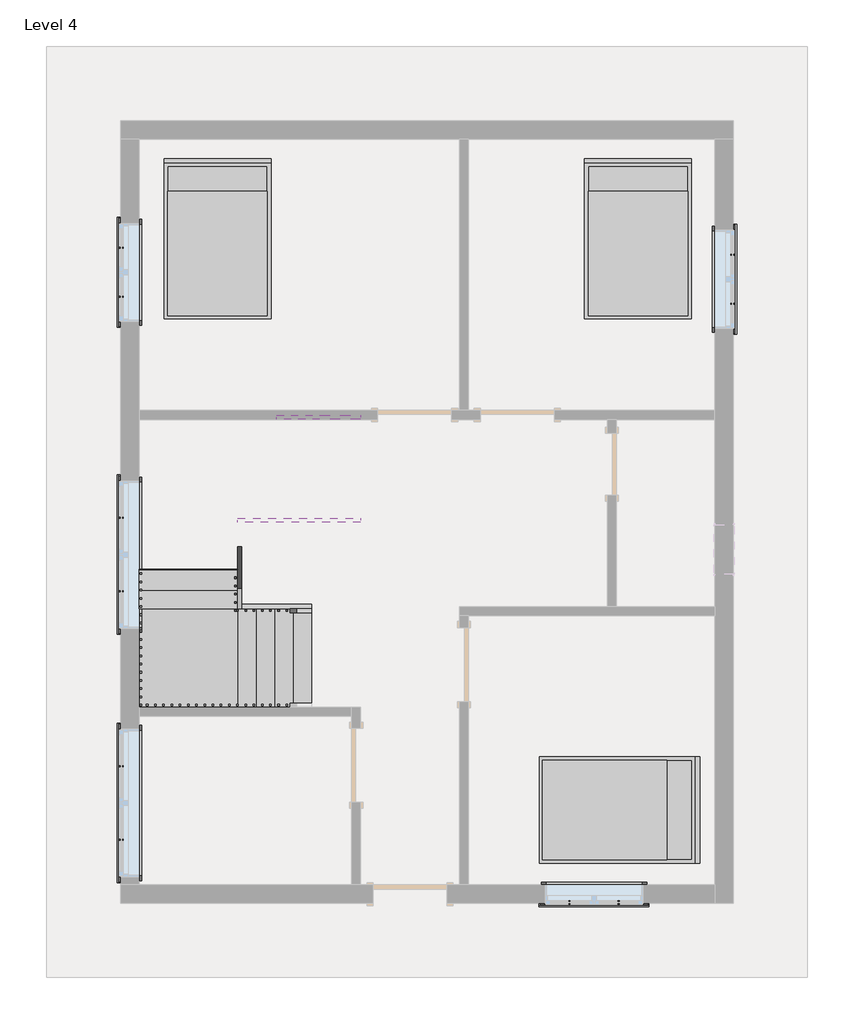
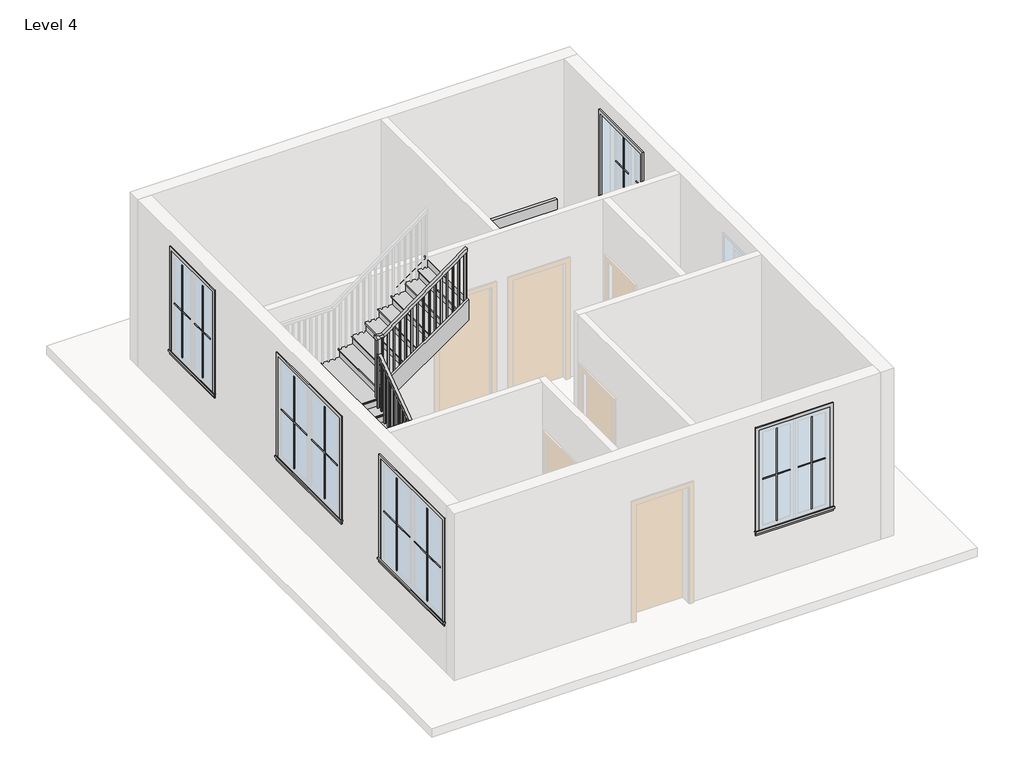
# One storey, part 3 of 3: 20 proxies, 5 members, 3 furniture elements, 1 railing, 1 stair flight.
"""IFC4 building model written with IfcOpenShell, lengths in millimetres."""

from ifc_helpers import new_model, si_unit, frame, origin, place, context, project, spatial, polyline, outline, extrude, faceted_brep, transform, mapped, element, save
from components import muntin_pattern_2x2_muntin_pattern_2x2_0a037076, muntin_pattern_2x2_muntin_pattern_2x2_e6f69628, muntin_pattern_2x2_muntin_pattern_2x2_2b4d9f72, muntin_pattern_2x2_muntin_pattern_2x2_ef995ed3, trim_window_exterior_flat_with_sill_b601e94a, trim_window_exterior_flat_with_sill_b7e4d11c, trim_window_interior_flat_picture_frame_bfefb25c, trim_window_interior_flat_picture_frame_936b8d2a, bed_17739_bed_17739_15c61121, stair_flight_abd4a925

model = new_model("IFC4")

# Units and contexts
model_context = context("Model", 3, world=origin())
ifc_project = project(units=[si_unit("LENGTHUNIT", "METRE", prefix="MILLI")], contexts=[model_context])

# Site, building, storey
site = spatial("IfcSite", under=ifc_project)
building = spatial("IfcBuilding", under=site)
storey = spatial("IfcBuildingStorey", under=building, Name="Level 4", Elevation=9448.8)

# Proxies
placement = place(None, origin())
muntin_pattern_2x2_muntin_pattern_2x2_shape = muntin_pattern_2x2_muntin_pattern_2x2_0a037076(model_context)
element("IfcBuildingElementProxy", 1, Name="Muntin Pattern_2x2 : Muntin Pattern_2x2", ObjectType="Muntin Pattern_2x2 : Muntin Pattern_2x2", at=placement, inside=storey, context=model_context, shape_type="MappedRepresentation", body=[
    mapped(muntin_pattern_2x2_muntin_pattern_2x2_shape, transform((-5035.7855391, -4380.9248761, 10433.05), x_axis=(0.0, 1.0, 0.0), y_axis=(-1.0, 0.0, 0.0), z_axis=(0.0, 0.0, 1.0))),
])
element("IfcBuildingElementProxy", 2, Name="Muntin Pattern_2x2 : Muntin Pattern_2x2", ObjectType="Muntin Pattern_2x2 : Muntin Pattern_2x2", at=placement, inside=storey, context=model_context, shape_type="MappedRepresentation", body=[
    mapped(muntin_pattern_2x2_muntin_pattern_2x2_shape, transform((-5035.7855391, -1310.6998761, 10433.05), x_axis=(0.0, 1.0, 0.0), y_axis=(-1.0, 0.0, 0.0), z_axis=(0.0, 0.0, 1.0))),
])
muntin_pattern_2x2_muntin_pattern_2x2_2_shape = muntin_pattern_2x2_muntin_pattern_2x2_e6f69628(model_context)
element("IfcBuildingElementProxy", 3, Name="Muntin Pattern_2x2 : Muntin Pattern_2x2", ObjectType="Muntin Pattern_2x2 : Muntin Pattern_2x2", at=placement, inside=storey, context=model_context, shape_type="MappedRepresentation", body=[
    mapped(muntin_pattern_2x2_muntin_pattern_2x2_2_shape, transform((-5035.7855391, -3469.6998761, 10433.05), x_axis=(0.0, -1.0, 0.0), y_axis=(1.0, 0.0, 0.0), z_axis=(0.0, 0.0, 1.0))),
])
element("IfcBuildingElementProxy", 4, Name="Muntin Pattern_2x2 : Muntin Pattern_2x2", ObjectType="Muntin Pattern_2x2 : Muntin Pattern_2x2", at=placement, inside=storey, context=model_context, shape_type="MappedRepresentation", body=[
    mapped(muntin_pattern_2x2_muntin_pattern_2x2_2_shape, transform((-5035.7855391, -399.4748761, 10433.05), x_axis=(0.0, -1.0, 0.0), y_axis=(1.0, 0.0, 0.0), z_axis=(0.0, 0.0, 1.0))),
])
muntin_pattern_2x2_muntin_pattern_2x2_3_shape = muntin_pattern_2x2_muntin_pattern_2x2_2b4d9f72(model_context)
element("IfcBuildingElementProxy", 5, Name="Muntin Pattern_2x2 : Muntin Pattern_2x2", ObjectType="Muntin Pattern_2x2 : Muntin Pattern_2x2", at=placement, inside=storey, context=model_context, shape_type="MappedRepresentation", body=[
    mapped(muntin_pattern_2x2_muntin_pattern_2x2_3_shape, transform((1115.7769609, -5157.2123761, 10433.05), x_axis=(-1.0, 0.0, 0.0), y_axis=(0.0, -1.0, 0.0), z_axis=(0.0, 0.0, 1.0))),
])
element("IfcBuildingElementProxy", 6, Name="Muntin Pattern_2x2 : Muntin Pattern_2x2", ObjectType="Muntin Pattern_2x2 : Muntin Pattern_2x2", at=placement, inside=storey, context=model_context, shape_type="MappedRepresentation", body=[
    mapped(muntin_pattern_2x2_muntin_pattern_2x2_3_shape, transform((2527.0644609, 2851.7251239, 10433.05), x_axis=(0.0, -1.0, 0.0), y_axis=(1.0, 0.0, 0.0), z_axis=(0.0, 0.0, 1.0))),
])
element("IfcBuildingElementProxy", 7, Name="Muntin Pattern_2x2 : Muntin Pattern_2x2", ObjectType="Muntin Pattern_2x2 : Muntin Pattern_2x2", at=placement, inside=storey, context=model_context, shape_type="MappedRepresentation", body=[
    mapped(muntin_pattern_2x2_muntin_pattern_2x2_3_shape, transform((-5035.7855391, 2331.0251239, 10433.05), x_axis=(0.0, 1.0, 0.0), y_axis=(-1.0, 0.0, 0.0), z_axis=(0.0, 0.0, 1.0))),
])
muntin_pattern_2x2_muntin_pattern_2x2_4_shape = muntin_pattern_2x2_muntin_pattern_2x2_ef995ed3(model_context)
element("IfcBuildingElementProxy", 8, Name="Muntin Pattern_2x2 : Muntin Pattern_2x2", ObjectType="Muntin Pattern_2x2 : Muntin Pattern_2x2", at=placement, inside=storey, context=model_context, shape_type="MappedRepresentation", body=[
    mapped(muntin_pattern_2x2_muntin_pattern_2x2_4_shape, transform((509.3519609, -5157.2123761, 10433.05), x_axis=(1.0, 0.0, 0.0), y_axis=(0.0, 1.0, 0.0), z_axis=(0.0, 0.0, 1.0))),
])
element("IfcBuildingElementProxy", 9, Name="Muntin Pattern_2x2 : Muntin Pattern_2x2", ObjectType="Muntin Pattern_2x2 : Muntin Pattern_2x2", at=placement, inside=storey, context=model_context, shape_type="MappedRepresentation", body=[
    mapped(muntin_pattern_2x2_muntin_pattern_2x2_4_shape, transform((2527.0644609, 2245.3001239, 10433.05), x_axis=(0.0, 1.0, 0.0), y_axis=(-1.0, 0.0, 0.0), z_axis=(0.0, 0.0, 1.0))),
])
element("IfcBuildingElementProxy", 10, Name="Muntin Pattern_2x2 : Muntin Pattern_2x2", ObjectType="Muntin Pattern_2x2 : Muntin Pattern_2x2", at=placement, inside=storey, context=model_context, shape_type="MappedRepresentation", body=[
    mapped(muntin_pattern_2x2_muntin_pattern_2x2_4_shape, transform((-5035.7855391, 2937.4501239, 10433.05), x_axis=(0.0, -1.0, 0.0), y_axis=(1.0, 0.0, 0.0), z_axis=(0.0, 0.0, 1.0))),
])
trim_window_exterior_flat_with_sill_shape = trim_window_exterior_flat_with_sill_b601e94a(model_context)
element("IfcBuildingElementProxy", 11, Name="Trim-Window-Exterior-Flat : with Sill", ObjectType="Trim-Window-Exterior-Flat : with Sill", at=placement, inside=storey, context=model_context, shape_type="MappedRepresentation", body=[
    mapped(trim_window_exterior_flat_with_sill_shape, transform((-5045.3105391, -3925.3123761, 12192.0), x_axis=(0.0, -1.0, 0.0), y_axis=(0.0, 0.0, 1.0), z_axis=(-1.0, 0.0, 0.0))),
])
element("IfcBuildingElementProxy", 12, Name="Trim-Window-Exterior-Flat : with Sill", ObjectType="Trim-Window-Exterior-Flat : with Sill", at=placement, inside=storey, context=model_context, shape_type="MappedRepresentation", body=[
    mapped(trim_window_exterior_flat_with_sill_shape, transform((-5045.3105391, -855.0873761, 12192.0), x_axis=(0.0, -1.0, 0.0), y_axis=(0.0, 0.0, 1.0), z_axis=(-1.0, 0.0, 0.0))),
])
trim_window_exterior_flat_with_sill_2_shape = trim_window_exterior_flat_with_sill_b7e4d11c(model_context)
element("IfcBuildingElementProxy", 13, Name="Trim-Window-Exterior-Flat : with Sill", ObjectType="Trim-Window-Exterior-Flat : with Sill", at=placement, inside=storey, context=model_context, shape_type="MappedRepresentation", body=[
    mapped(trim_window_exterior_flat_with_sill_2_shape, transform((812.5644609, -5166.7373761, 12192.0), x_axis=(1.0, 0.0, 0.0), y_axis=(0.0, 0.0, 1.0), z_axis=(0.0, -1.0, 0.0))),
])
element("IfcBuildingElementProxy", 14, Name="Trim-Window-Exterior-Flat : with Sill", ObjectType="Trim-Window-Exterior-Flat : with Sill", at=placement, inside=storey, context=model_context, shape_type="MappedRepresentation", body=[
    mapped(trim_window_exterior_flat_with_sill_2_shape, transform((2536.5894609, 2548.5126239, 12192.0), x_axis=(0.0, 1.0, 0.0), y_axis=(0.0, 0.0, 1.0), z_axis=(1.0, 0.0, 0.0))),
])
element("IfcBuildingElementProxy", 15, Name="Trim-Window-Exterior-Flat : with Sill", ObjectType="Trim-Window-Exterior-Flat : with Sill", at=placement, inside=storey, context=model_context, shape_type="MappedRepresentation", body=[
    mapped(trim_window_exterior_flat_with_sill_2_shape, transform((-5045.3105391, 2634.2376239, 12192.0), x_axis=(0.0, -1.0, 0.0), y_axis=(0.0, 0.0, 1.0), z_axis=(-1.0, 0.0, 0.0))),
])
trim_window_interior_flat_picture_frame_shape = trim_window_interior_flat_picture_frame_bfefb25c(model_context)
element("IfcBuildingElementProxy", 16, Name="Trim-Window-Interior-Flat : Picture Frame", ObjectType="Trim-Window-Interior-Flat : Picture Frame", at=placement, inside=storey, context=model_context, shape_type="MappedRepresentation", body=[
    mapped(trim_window_interior_flat_picture_frame_shape, transform((-4816.7105391, -3925.3123761, 12192.0), x_axis=(0.0, 1.0, 0.0), y_axis=(0.0, 0.0, 1.0), z_axis=(1.0, 0.0, 0.0))),
])
element("IfcBuildingElementProxy", 17, Name="Trim-Window-Interior-Flat : Picture Frame", ObjectType="Trim-Window-Interior-Flat : Picture Frame", at=placement, inside=storey, context=model_context, shape_type="MappedRepresentation", body=[
    mapped(trim_window_interior_flat_picture_frame_shape, transform((-4816.7105391, -855.0873761, 12192.0), x_axis=(0.0, 1.0, 0.0), y_axis=(0.0, 0.0, 1.0), z_axis=(1.0, 0.0, 0.0))),
])
trim_window_interior_flat_picture_frame_2_shape = trim_window_interior_flat_picture_frame_936b8d2a(model_context)
element("IfcBuildingElementProxy", 18, Name="Trim-Window-Interior-Flat : Picture Frame", ObjectType="Trim-Window-Interior-Flat : Picture Frame", at=placement, inside=storey, context=model_context, shape_type="MappedRepresentation", body=[
    mapped(trim_window_interior_flat_picture_frame_2_shape, transform((812.5644609, -4938.1373761, 12192.0), x_axis=(-1.0, 0.0, 0.0), y_axis=(0.0, 0.0, 1.0), z_axis=(0.0, 1.0, 0.0))),
])
element("IfcBuildingElementProxy", 19, Name="Trim-Window-Interior-Flat : Picture Frame", ObjectType="Trim-Window-Interior-Flat : Picture Frame", at=placement, inside=storey, context=model_context, shape_type="MappedRepresentation", body=[
    mapped(trim_window_interior_flat_picture_frame_2_shape, transform((2307.9894609, 2548.5126239, 12192.0), x_axis=(0.0, -1.0, 0.0), y_axis=(0.0, 0.0, 1.0), z_axis=(-1.0, 0.0, 0.0))),
])
element("IfcBuildingElementProxy", 20, Name="Trim-Window-Interior-Flat : Picture Frame", ObjectType="Trim-Window-Interior-Flat : Picture Frame", at=placement, inside=storey, context=model_context, shape_type="MappedRepresentation", body=[
    mapped(trim_window_interior_flat_picture_frame_2_shape, transform((-4816.7105391, 2634.2376239, 12192.0), x_axis=(0.0, 1.0, 0.0), y_axis=(0.0, 0.0, 1.0), z_axis=(1.0, 0.0, 0.0))),
])

# Furniture
bed_17739_bed_17739_shape = bed_17739_bed_17739_15c61121(model_context)
element("IfcFurniture", 21, ObjectType="Bed_17739 : Bed_17739", at=placement, inside=storey, context=model_context, shape_type="MappedRepresentation", body=[
    mapped(bed_17739_bed_17739_shape, transform((-3845.1605391, 3024.7626239, 9448.8), x_axis=(1.0, 0.0, 0.0), y_axis=(0.0, 1.0, 0.0), z_axis=(0.0, 0.0, 1.0))),
])
element("IfcFurniture", 22, ObjectType="Bed_17739 : Bed_17739", at=placement, inside=storey, context=model_context, shape_type="MappedRepresentation", body=[
    mapped(bed_17739_bed_17739_shape, transform((1355.4894609, 3024.7626239, 9448.8), x_axis=(1.0, 0.0, 0.0), y_axis=(0.0, 1.0, 0.0), z_axis=(0.0, 0.0, 1.0))),
])
element("IfcFurniture", 23, ObjectType="Bed_17739 : Bed_17739", at=placement, inside=storey, context=model_context, shape_type="MappedRepresentation", body=[
    mapped(bed_17739_bed_17739_shape, transform((1101.4894609, -4011.0373761, 9448.8), x_axis=(0.0, -1.0, 0.0), y_axis=(1.0, 0.0, 0.0), z_axis=(0.0, 0.0, 1.0))),
])

# Members
element("IfcMember", 24, ObjectType="Stringer - 2\" Width", at=placement, inside=storey, context=model_context, shape_type="SweptSolid", body=[
    extrude(outline(polyline([(9448.8, -2683.1105391), (9599.3087903, -2683.1105391), (9599.3087903, -3112.2707489), (9448.8, -2897.7957228), (9448.8, -2683.1105391)])), frame((0.0, -2791.8373761, 0.0), z_axis=(0.0, 1.0, 0.0), x_axis=(0.0, 0.0, 1.0)), (0.0, 0.0, 1.0), 50.8),
])
element("IfcMember", 25, ObjectType="Stringer - 2\" Width", at=placement, inside=storey, context=model_context, shape_type="SweptSolid", body=[
    extrude(outline(polyline([(11776.2856495, -2580.7583047), (12132.2489938, -2073.5105391), (12504.6117181, -2073.5105391), (11776.2856495, -3111.3751869), (11776.2856495, -2580.7583047)])), frame((0.0, 814.9626239, 0.0), z_axis=(0.0, 1.0, 0.0), x_axis=(0.0, 0.0, 1.0)), (0.0, 0.0, 1.0), 50.8),
])
element("IfcMember", 26, ObjectType="Stringer - 2\" Width", at=placement, inside=storey, context=model_context, shape_type="SweptSolid", body=[
    extrude(outline(polyline([(9448.8, -2683.1105391), (9670.506455, -2683.1105391), (10276.5415427, -3546.7105391), (9904.1788184, -3546.7105391), (9448.8, -2897.7957228), (9448.8, -2683.1105391)])), frame((0.0, -1521.8373761, 0.0), z_axis=(0.0, 1.0, 0.0), x_axis=(0.0, 0.0, 1.0)), (0.0, 0.0, 1.0), 50.8),
])
element("IfcMember", 27, ObjectType="Stringer - 2\" Width", at=placement, inside=storey, context=model_context, shape_type="SweptSolid", body=[
    extrude(outline(polyline([(-1521.8373761, 10099.1564629), (-1521.8373761, 10474.3327137), (-455.0373761, 11239.9786467), (-455.0373761, 10864.8023959), (-1521.8373761, 10099.1564629)])), frame((-3597.5105391, 0.0, 0.0), z_axis=(1.0, 0.0, 0.0), x_axis=(0.0, 1.0, 0.0)), (0.0, 0.0, 1.0), 50.8),
])
element("IfcMember", 28, ObjectType="Stringer - 2\" Width", at=placement, inside=storey, context=model_context, shape_type="SweptSolid", body=[
    extrude(outline(polyline([(11435.1380339, -3597.5105391), (11062.7753096, -3597.5105391), (12132.2489938, -2073.5105391), (12504.6117181, -2073.5105391), (11435.1380339, -3597.5105391)])), frame((0.0, -455.0373761, 0.0), z_axis=(0.0, 1.0, 0.0), x_axis=(0.0, 0.0, 1.0)), (0.0, 0.0, 1.0), 50.8),
])

# Railing
element("IfcRailing", 29, ObjectType="Handrail - Rectangular", at=placement, inside=storey, context=model_context, shape_type="SolidModel", body=[
    faceted_brep([(-2683.1105391, -1572.6373761, 10523.6210526), (-2683.1105391, -1572.6373761, 10461.5605986), (-2683.1105391, -1521.8373761, 10461.5605986), (-2683.1105391, -1521.8373761, 10523.6210526), (-3521.3105391, -1572.6373761, 11111.8315789), (-3572.1105391, -1572.6373761, 11085.4202477), (-3572.1105391, -1521.8373761, 11085.4202477), (-3521.3105391, -1521.8373761, 11111.8315789), (-3521.3105391, -1572.6373761, 11380.415311), (-3572.1105391, -1572.6373761, 11329.615311), (-3572.1105391, -1521.8373761, 11329.615311), (-3521.3105391, -1521.8373761, 11380.415311), (-3648.3105391, -1572.6373761, 11380.415311), (-3648.3105391, -1572.6373761, 11329.615311), (-3597.5105391, -1521.8373761, 11329.615311), (-3597.5105391, -1521.8373761, 11380.415311), (-3648.3105391, -1445.6373761, 11380.415311), (-3648.3105391, -1429.2944467, 11329.615311), (-3597.5105391, -1429.2944467, 11329.615311), (-3597.5105391, -1445.6373761, 11380.415311), (-3648.3105391, -480.4373761, 12073.1425837), (-3648.3105391, -429.6373761, 12047.0725387), (-3597.5105391, -429.6373761, 12047.0725387), (-3597.5105391, -480.4373761, 12073.1425837), (-3648.3105391, -480.4373761, 12344.4), (-3648.3105391, -429.6373761, 12293.6), (-3597.5105391, -429.6373761, 12293.6), (-3597.5105391, -480.4373761, 12344.4), (-3648.3105391, -353.4373761, 12344.4), (-3648.3105391, -353.4373761, 12293.6), (-3597.5105391, -404.2373761, 12293.6), (-3597.5105391, -404.2373761, 12344.4), (-3521.3105391, -353.4373761, 12344.4), (-3504.6160355, -353.4373761, 12293.6), (-3504.6160355, -404.2373761, 12293.6), (-3521.3105391, -404.2373761, 12344.4), (-2073.5105391, -353.4373761, 13411.2), (-2073.5105391, -404.2373761, 13411.2), (-2073.5105391, -404.2373761, 13348.0987868), (-2073.5105391, -353.4373761, 13348.0987868)], [[[0, 1, 2, 3]], [[1, 0, 4, 5]], [[2, 1, 5, 6]], [[3, 2, 6, 7]], [[0, 3, 7, 4]], [[5, 4, 8, 9]], [[6, 5, 9, 10]], [[7, 6, 10, 11]], [[4, 7, 11, 8]], [[9, 8, 12, 13]], [[10, 9, 13, 14]], [[11, 10, 14, 15]], [[8, 11, 15, 12]], [[13, 12, 16, 17]], [[14, 13, 17, 18]], [[15, 14, 18, 19]], [[12, 15, 19, 16]], [[17, 16, 20, 21]], [[18, 17, 21, 22]], [[19, 18, 22, 23]], [[16, 19, 23, 20]], [[21, 20, 24, 25]], [[22, 21, 25, 26]], [[23, 22, 26, 27]], [[20, 23, 27, 24]], [[25, 24, 28, 29]], [[26, 25, 29, 30]], [[27, 26, 30, 31]], [[24, 27, 31, 28]], [[29, 28, 32, 33]], [[30, 29, 33, 34]], [[31, 30, 34, 35]], [[28, 31, 35, 32]], [[36, 37, 38, 39]], [[33, 32, 36, 39]], [[34, 33, 39, 38]], [[35, 34, 38, 37]], [[32, 35, 37, 36]]]),
    extrude(outline(polyline([(13336.4014184, -2089.3855391), (13322.3645763, -2108.4355391), (12336.3789474, -2108.4355391), (12336.3789474, -2089.3855391), (13336.4014184, -2089.3855391)])), frame((0.0, -388.3623761, 0.0), z_axis=(0.0, 1.0, 0.0), x_axis=(0.0, 0.0, 1.0)), (0.0, 0.0, 1.0), 19.05),
    extrude(outline(polyline([(13261.5382605, -2190.9855391), (13247.5014184, -2210.0355391), (12336.3789474, -2210.0355391), (12336.3789474, -2190.9855391), (13261.5382605, -2190.9855391)])), frame((0.0, -388.3623761, 0.0), z_axis=(0.0, 1.0, 0.0), x_axis=(0.0, 0.0, 1.0)), (0.0, 0.0, 1.0), 19.05),
    extrude(outline(polyline([(13186.6751026, -2292.5855391), (13172.6382605, -2311.6355391), (12175.9578947, -2311.6355391), (12175.9578947, -2292.5855391), (13186.6751026, -2292.5855391)])), frame((0.0, -388.3623761, 0.0), z_axis=(0.0, 1.0, 0.0), x_axis=(0.0, 0.0, 1.0)), (0.0, 0.0, 1.0), 19.05),
    extrude(outline(polyline([(13111.8119447, -2394.1855391), (13097.7751026, -2413.2355391), (12175.9578947, -2413.2355391), (12175.9578947, -2394.1855391), (13111.8119447, -2394.1855391)])), frame((0.0, -388.3623761, 0.0), z_axis=(0.0, 1.0, 0.0), x_axis=(0.0, 0.0, 1.0)), (0.0, 0.0, 1.0), 19.05),
    extrude(outline(polyline([(13036.9487868, -2495.7855391), (13022.9119447, -2514.8355391), (12015.5368421, -2514.8355391), (12015.5368421, -2495.7855391), (13036.9487868, -2495.7855391)])), frame((0.0, -388.3623761, 0.0), z_axis=(0.0, 1.0, 0.0), x_axis=(0.0, 0.0, 1.0)), (0.0, 0.0, 1.0), 19.05),
    extrude(outline(polyline([(12962.0856289, -2597.3855391), (12948.0487868, -2616.4355391), (12015.5368421, -2616.4355391), (12015.5368421, -2597.3855391), (12962.0856289, -2597.3855391)])), frame((0.0, -388.3623761, 0.0), z_axis=(0.0, 1.0, 0.0), x_axis=(0.0, 0.0, 1.0)), (0.0, 0.0, 1.0), 19.05),
    extrude(outline(polyline([(12887.222471, -2698.9855391), (12873.1856289, -2718.0355391), (11855.1157895, -2718.0355391), (11855.1157895, -2698.9855391), (12887.222471, -2698.9855391)])), frame((0.0, -388.3623761, 0.0), z_axis=(0.0, 1.0, 0.0), x_axis=(0.0, 0.0, 1.0)), (0.0, 0.0, 1.0), 19.05),
    extrude(outline(polyline([(12812.3593132, -2800.5855391), (12798.322471, -2819.6355391), (11855.1157895, -2819.6355391), (11855.1157895, -2800.5855391), (12812.3593132, -2800.5855391)])), frame((0.0, -388.3623761, 0.0), z_axis=(0.0, 1.0, 0.0), x_axis=(0.0, 0.0, 1.0)), (0.0, 0.0, 1.0), 19.05),
    extrude(outline(polyline([(12737.4961553, -2902.1855391), (12723.4593132, -2921.2355391), (11855.1157895, -2921.2355391), (11855.1157895, -2902.1855391), (12737.4961553, -2902.1855391)])), frame((0.0, -388.3623761, 0.0), z_axis=(0.0, 1.0, 0.0), x_axis=(0.0, 0.0, 1.0)), (0.0, 0.0, 1.0), 19.05),
    extrude(outline(polyline([(12662.6329974, -3003.7855391), (12648.5961553, -3022.8355391), (11694.6947368, -3022.8355391), (11694.6947368, -3003.7855391), (12662.6329974, -3003.7855391)])), frame((0.0, -388.3623761, 0.0), z_axis=(0.0, 1.0, 0.0), x_axis=(0.0, 0.0, 1.0)), (0.0, 0.0, 1.0), 19.05),
    extrude(outline(polyline([(12587.7698395, -3105.3855391), (12573.7329974, -3124.4355391), (11694.6947368, -3124.4355391), (11694.6947368, -3105.3855391), (12587.7698395, -3105.3855391)])), frame((0.0, -388.3623761, 0.0), z_axis=(0.0, 1.0, 0.0), x_axis=(0.0, 0.0, 1.0)), (0.0, 0.0, 1.0), 19.05),
    extrude(outline(polyline([(12512.9066816, -3206.9855391), (12498.8698395, -3226.0355391), (11534.2736842, -3226.0355391), (11534.2736842, -3206.9855391), (12512.9066816, -3206.9855391)])), frame((0.0, -388.3623761, 0.0), z_axis=(0.0, 1.0, 0.0), x_axis=(0.0, 0.0, 1.0)), (0.0, 0.0, 1.0), 19.05),
    extrude(outline(polyline([(12438.0435237, -3308.5855391), (12424.0066816, -3327.6355391), (11534.2736842, -3327.6355391), (11534.2736842, -3308.5855391), (12438.0435237, -3308.5855391)])), frame((0.0, -388.3623761, 0.0), z_axis=(0.0, 1.0, 0.0), x_axis=(0.0, 0.0, 1.0)), (0.0, 0.0, 1.0), 19.05),
    extrude(outline(polyline([(12363.1803658, -3410.1855391), (12349.1435237, -3429.2355391), (11373.8526316, -3429.2355391), (11373.8526316, -3410.1855391), (12363.1803658, -3410.1855391)])), frame((0.0, -388.3623761, 0.0), z_axis=(0.0, 1.0, 0.0), x_axis=(0.0, 0.0, 1.0)), (0.0, 0.0, 1.0), 19.05),
    extrude(outline(polyline([(12288.3172079, -3511.7855391), (12274.2803658, -3530.8355391), (11373.8526316, -3530.8355391), (11373.8526316, -3511.7855391), (12288.3172079, -3511.7855391)])), frame((0.0, -388.3623761, 0.0), z_axis=(0.0, 1.0, 0.0), x_axis=(0.0, 0.0, 1.0)), (0.0, 0.0, 1.0), 19.05),
    extrude(outline(polyline([(-3613.3855391, -439.1623761), (-3632.4355391, -439.1623761), (-3632.4355391, -420.1123761), (-3613.3855391, -420.1123761), (-3613.3855391, -439.1623761)])), frame((0.0, 0.0, 11053.0105263), z_axis=(0.0, 0.0, 1.0), x_axis=(1.0, 0.0, 0.0)), (0.0, 0.0, 1.0), 1240.5894737),
    extrude(outline(polyline([(-540.7623761, 11967.3177541), (-521.7123761, 11980.9900029), (-521.7123761, 11053.0105263), (-540.7623761, 11053.0105263), (-540.7623761, 11967.3177541)])), frame((-3632.4355391, 0.0, 0.0), z_axis=(1.0, 0.0, 0.0), x_axis=(0.0, 1.0, 0.0)), (0.0, 0.0, 1.0), 19.05),
    extrude(outline(polyline([(-642.3623761, 11894.3990938), (-623.3123761, 11908.0713426), (-623.3123761, 10892.5894737), (-642.3623761, 10892.5894737), (-642.3623761, 11894.3990938)])), frame((-3632.4355391, 0.0, 0.0), z_axis=(1.0, 0.0, 0.0), x_axis=(0.0, 1.0, 0.0)), (0.0, 0.0, 1.0), 19.05),
    extrude(outline(polyline([(-743.9623761, 11821.4804335), (-724.9123761, 11835.1526823), (-724.9123761, 10892.5894737), (-743.9623761, 10892.5894737), (-743.9623761, 11821.4804335)])), frame((-3632.4355391, 0.0, 0.0), z_axis=(1.0, 0.0, 0.0), x_axis=(0.0, 1.0, 0.0)), (0.0, 0.0, 1.0), 19.05),
    extrude(outline(polyline([(-845.5623761, 11748.5617732), (-826.5123761, 11762.234022), (-826.5123761, 10892.5894737), (-845.5623761, 10892.5894737), (-845.5623761, 11748.5617732)])), frame((-3632.4355391, 0.0, 0.0), z_axis=(1.0, 0.0, 0.0), x_axis=(0.0, 1.0, 0.0)), (0.0, 0.0, 1.0), 19.05),
    extrude(outline(polyline([(-947.1623761, 11675.6431129), (-928.1123761, 11689.3153617), (-928.1123761, 10732.1684211), (-947.1623761, 10732.1684211), (-947.1623761, 11675.6431129)])), frame((-3632.4355391, 0.0, 0.0), z_axis=(1.0, 0.0, 0.0), x_axis=(0.0, 1.0, 0.0)), (0.0, 0.0, 1.0), 19.05),
    extrude(outline(polyline([(-1048.7623761, 11602.7244526), (-1029.7123761, 11616.3967014), (-1029.7123761, 10732.1684211), (-1048.7623761, 10732.1684211), (-1048.7623761, 11602.7244526)])), frame((-3632.4355391, 0.0, 0.0), z_axis=(1.0, 0.0, 0.0), x_axis=(0.0, 1.0, 0.0)), (0.0, 0.0, 1.0), 19.05),
    extrude(outline(polyline([(-1150.3623761, 11529.8057923), (-1131.3123761, 11543.4780411), (-1131.3123761, 10571.7473684), (-1150.3623761, 10571.7473684), (-1150.3623761, 11529.8057923)])), frame((-3632.4355391, 0.0, 0.0), z_axis=(1.0, 0.0, 0.0), x_axis=(0.0, 1.0, 0.0)), (0.0, 0.0, 1.0), 19.05),
    extrude(outline(polyline([(-1251.9623761, 11456.887132), (-1232.9123761, 11470.5593808), (-1232.9123761, 10571.7473684), (-1251.9623761, 10571.7473684), (-1251.9623761, 11456.887132)])), frame((-3632.4355391, 0.0, 0.0), z_axis=(1.0, 0.0, 0.0), x_axis=(0.0, 1.0, 0.0)), (0.0, 0.0, 1.0), 19.05),
    extrude(outline(polyline([(-1353.5623761, 11383.9684718), (-1334.5123761, 11397.6407206), (-1334.5123761, 10411.3263158), (-1353.5623761, 10411.3263158), (-1353.5623761, 11383.9684718)])), frame((-3632.4355391, 0.0, 0.0), z_axis=(1.0, 0.0, 0.0), x_axis=(0.0, 1.0, 0.0)), (0.0, 0.0, 1.0), 19.05),
    extrude(outline(polyline([(-1455.1623761, 11311.0498115), (-1436.1123761, 11324.7220603), (-1436.1123761, 10411.3263158), (-1455.1623761, 10411.3263158), (-1455.1623761, 11311.0498115)])), frame((-3632.4355391, 0.0, 0.0), z_axis=(1.0, 0.0, 0.0), x_axis=(0.0, 1.0, 0.0)), (0.0, 0.0, 1.0), 19.05),
    extrude(outline(polyline([(-3587.9855391, -1537.7123761), (-3587.9855391, -1556.7623761), (-3607.0355391, -1556.7623761), (-3607.0355391, -1537.7123761), (-3587.9855391, -1537.7123761)])), frame((0.0, 0.0, 10250.9052632), z_axis=(0.0, 0.0, 1.0), x_axis=(1.0, 0.0, 0.0)), (0.0, 0.0, 1.0), 1078.7100478),
    extrude(outline(polyline([(11025.262353, -3486.3855391), (11038.630774, -3505.4355391), (10090.4842105, -3505.4355391), (10090.4842105, -3486.3855391), (11025.262353, -3486.3855391)])), frame((0.0, -1556.7623761, 0.0), z_axis=(0.0, 1.0, 0.0), x_axis=(0.0, 0.0, 1.0)), (0.0, 0.0, 1.0), 19.05),
    extrude(outline(polyline([(10953.9641074, -3384.7855391), (10967.3325284, -3403.8355391), (10090.4842105, -3403.8355391), (10090.4842105, -3384.7855391), (10953.9641074, -3384.7855391)])), frame((0.0, -1556.7623761, 0.0), z_axis=(0.0, 1.0, 0.0), x_axis=(0.0, 0.0, 1.0)), (0.0, 0.0, 1.0), 19.05),
    extrude(outline(polyline([(10882.6658617, -3283.1855391), (10896.0342828, -3302.2355391), (9930.0631579, -3302.2355391), (9930.0631579, -3283.1855391), (10882.6658617, -3283.1855391)])), frame((0.0, -1556.7623761, 0.0), z_axis=(0.0, 1.0, 0.0), x_axis=(0.0, 0.0, 1.0)), (0.0, 0.0, 1.0), 19.05),
    extrude(outline(polyline([(10811.3676161, -3181.5855391), (10824.7360372, -3200.6355391), (9930.0631579, -3200.6355391), (9930.0631579, -3181.5855391), (10811.3676161, -3181.5855391)])), frame((0.0, -1556.7623761, 0.0), z_axis=(0.0, 1.0, 0.0), x_axis=(0.0, 0.0, 1.0)), (0.0, 0.0, 1.0), 19.05),
    extrude(outline(polyline([(10740.0693705, -3079.9855391), (10753.4377916, -3099.0355391), (9769.6421053, -3099.0355391), (9769.6421053, -3079.9855391), (10740.0693705, -3079.9855391)])), frame((0.0, -1556.7623761, 0.0), z_axis=(0.0, 1.0, 0.0), x_axis=(0.0, 0.0, 1.0)), (0.0, 0.0, 1.0), 19.05),
    extrude(outline(polyline([(10668.7711249, -2978.3855391), (10682.1395459, -2997.4355391), (9769.6421053, -2997.4355391), (9769.6421053, -2978.3855391), (10668.7711249, -2978.3855391)])), frame((0.0, -1556.7623761, 0.0), z_axis=(0.0, 1.0, 0.0), x_axis=(0.0, 0.0, 1.0)), (0.0, 0.0, 1.0), 19.05),
    extrude(outline(polyline([(10597.4728793, -2876.7855391), (10610.8413003, -2895.8355391), (9609.2210526, -2895.8355391), (9609.2210526, -2876.7855391), (10597.4728793, -2876.7855391)])), frame((0.0, -1556.7623761, 0.0), z_axis=(0.0, 1.0, 0.0), x_axis=(0.0, 0.0, 1.0)), (0.0, 0.0, 1.0), 19.05),
    extrude(outline(polyline([(10526.1746337, -2775.1855391), (10539.5430547, -2794.2355391), (9609.2210526, -2794.2355391), (9609.2210526, -2775.1855391), (10526.1746337, -2775.1855391)])), frame((0.0, -1556.7623761, 0.0), z_axis=(0.0, 1.0, 0.0), x_axis=(0.0, 0.0, 1.0)), (0.0, 0.0, 1.0), 19.05),
    extrude(outline(polyline([(-3613.3855391, -388.3623761), (-3632.4355391, -388.3623761), (-3632.4355391, -369.3123761), (-3613.3855391, -369.3123761), (-3613.3855391, -388.3623761)])), frame((0.0, 0.0, 11213.4315789), z_axis=(0.0, 0.0, 1.0), x_axis=(1.0, 0.0, 0.0)), (0.0, 0.0, 1.0), 1080.1684211),
    extrude(outline(polyline([(-3613.3855391, -1537.7123761), (-3613.3855391, -1556.7623761), (-3632.4355391, -1556.7623761), (-3632.4355391, -1537.7123761), (-3613.3855391, -1537.7123761)])), frame((0.0, 0.0, 10250.9052632), z_axis=(0.0, 0.0, 1.0), x_axis=(1.0, 0.0, 0.0)), (0.0, 0.0, 1.0), 1078.7100478),
    extrude(outline(polyline([(13348.0987868, -2073.5105391), (13334.0619447, -2092.5605391), (12336.3789474, -2092.5605391), (12336.3789474, -2073.5105391), (13348.0987868, -2073.5105391)])), frame((0.0, -388.3623761, 0.0), z_axis=(0.0, 1.0, 0.0), x_axis=(0.0, 0.0, 1.0)), (0.0, 0.0, 1.0), 19.05),
    extrude(outline(polyline([(10461.5605986, -2683.1105391), (10474.9290196, -2702.1605391), (9609.2210526, -2702.1605391), (9609.2210526, -2683.1105391), (10461.5605986, -2683.1105391)])), frame((0.0, -1556.7623761, 0.0), z_axis=(0.0, 1.0, 0.0), x_axis=(0.0, 0.0, 1.0)), (0.0, 0.0, 1.0), 19.05),
])

# Stair flight
stair_flight_shape = stair_flight_abd4a925(model_context)
element("IfcStairFlight", 30, ObjectType="2\" Tread 1\" Nosing 1/4\" Riser", at=placement, inside=storey, context=model_context, shape_type="MappedRepresentation", body=[
    mapped(stair_flight_shape, transform((0.0, 0.0, 0.0), x_axis=(1.0, 0.0, 0.0), y_axis=(0.0, 1.0, 0.0), z_axis=(0.0, 0.0, 1.0))),
])

save(model, "model.ifc")

# Revit data of these elements
# Type "Muntin Pattern_2x2 : Muntin Pattern_2x2"
#   Width [instance default] = 4' - 0"
#   Thickness = 0' - 0 1/2"
#   Height [instance default] = 4' - 0"
#   Distance = 0' - 0 3/4"
#   Interior Material [instance default] = none
#   Exterior Material [instance default] = none
#   Default Elevation = 0
# Type "Trim-Window-Exterior-Flat : with Sill"
#   Trim Width = 0' - 2 1/4"
#   Trim Thickness_Picture Frame = 0' - 1 1/4"
#   Trim Thickness_with Sill = 0' - 0 3/4"
#   Sill Thickness = 0' - 1 1/4"
#   Opening Width [instance default] = 2' - 0"
#   Opening Height [instance default] = 3' - 0"
#   Default Elevation = 4' - 0"
#   Sill = yes
#   Picture Frame = no
#   Trim Material [instance default] = none
# Type "Trim-Window-Interior-Flat : Picture Frame"
#   Trim Thickness_Picture Frame = 0' - 1 1/4"
#   Trim Width = 0' - 2 1/4"
#   Trim Thickness_with Sill = 0' - 0 3/4"
#   Sill Thickness = 0' - 1 1/4"
#   Opening Width [instance default] = 2' - 0"
#   Opening Height [instance default] = 3' - 0"
#   Default Elevation = 4' - 0"
#   Sill = no
#   Picture Frame = yes
#   Trim Material [instance default] = none
# Type "Bed_17739 : Bed_17739"
#   Default Elevation = 0
# Type "Handrail - Rectangular"
#   Assembly Code = "C2010400"
#   built-in parameter 1008612 = 0.0416667 (stored number, unit not read)
#   built-in parameter 1008611 = 0.0416667 (stored number, unit not read)
#   built-in parameter 1008609 = 0.333333 (stored number, unit not read)
#   built-in parameter 1008604 = 0.166667 (stored number, unit not read)
#   built-in parameter 1008603 = 0.166667 (stored number, unit not read)
#   Railing Height = 3' - 0"
#   built-in parameter 1008630 = 2
#   built-in parameter 1008610 = 2
#   built-in parameter 1008618 = Baluster - Square : 3/4"
# Elements 1, 2, 3, 4 (IfcBuildingElementProxy, "Muntin Pattern_2x2 : Muntin Pattern_2x2")
#   Width = 2' - 6 5/8"
#   Height = 5' - 6 1/2"
#   Interior Material = Wood - Stained
#   Exterior Material = Clad - White
#   Phase Created = New Construction
#   Materials on its faces: "Clad - White", "Wood - Stained"
# Elements 5, 6, 7, 8, 9, 10 (IfcBuildingElementProxy, "Muntin Pattern_2x2 : Muntin Pattern_2x2")
#   Width = 1' - 6 5/8"
#   Height = 5' - 6 1/2"
#   Interior Material = Wood - Stained
#   Exterior Material = Clad - White
#   Phase Created = New Construction
#   Materials on its faces: "Clad - White", "Wood - Stained"
# Elements 11, 12 (IfcBuildingElementProxy, "Trim-Window-Exterior-Flat : with Sill")
#   Opening Width = 6' - 0"
#   Opening Height = 6' - 0"
#   Trim Material = Clad - White
#   Phase Created = New Construction
#   Materials on its faces: "Clad - White"
# Elements 13, 14, 15 (IfcBuildingElementProxy, "Trim-Window-Exterior-Flat : with Sill")
#   Opening Width = 4' - 0"
#   Opening Height = 6' - 0"
#   Trim Material = Clad - White
#   Phase Created = New Construction
#   Materials on its faces: "Clad - White"
# Elements 16, 17 (IfcBuildingElementProxy, "Trim-Window-Interior-Flat : Picture Frame")
#   Opening Width = 6' - 0"
#   Opening Height = 6' - 0"
#   Trim Material = Wood - Stained
#   Phase Created = New Construction
#   Materials on its faces: "Wood - Stained"
# Elements 18, 19, 20 (IfcBuildingElementProxy, "Trim-Window-Interior-Flat : Picture Frame")
#   Opening Width = 4' - 0"
#   Opening Height = 6' - 0"
#   Trim Material = Wood - Stained
#   Phase Created = New Construction
#   Materials on its faces: "Wood - Stained"
# Elements 21, 22, 23 (IfcFurniture, "Bed_17739 : Bed_17739")
#   Phase Created = New Construction
#   Materials on its faces: "legs", "sheets", "bed frame", "Blanket"
# Elements 24, 25, 26, 27, 28 (IfcMember, "Stringer - 2\" Width")
#   Phase Created = New Construction
# Element 29 (IfcRailing, "Handrail - Rectangular")
#   Phase Created = New Construction
# Element 30 (IfcStairFlight, "2\" Tread 1\" Nosing 1/4\" Riser")
#   Phase Created = New Construction
# Materials
#   "Clad - White": class "Wood", colour RGB 242 242 238, transparency 0, Cost = 0
#   "Wood - Stained": class "Wood", colour RGB 224 178 126, transparency 0, Cost = 0
#   "legs": colour RGB 90 73 37, transparency 0, Cost = 0
#   "sheets": colour RGB 200 195 176, transparency 0, Cost = 0
#   "bed frame": colour RGB 90 73 37, transparency 0, Cost = 0
#   "Blanket": class "System", colour RGB 59 0 1, transparency 0, Cost = 0
